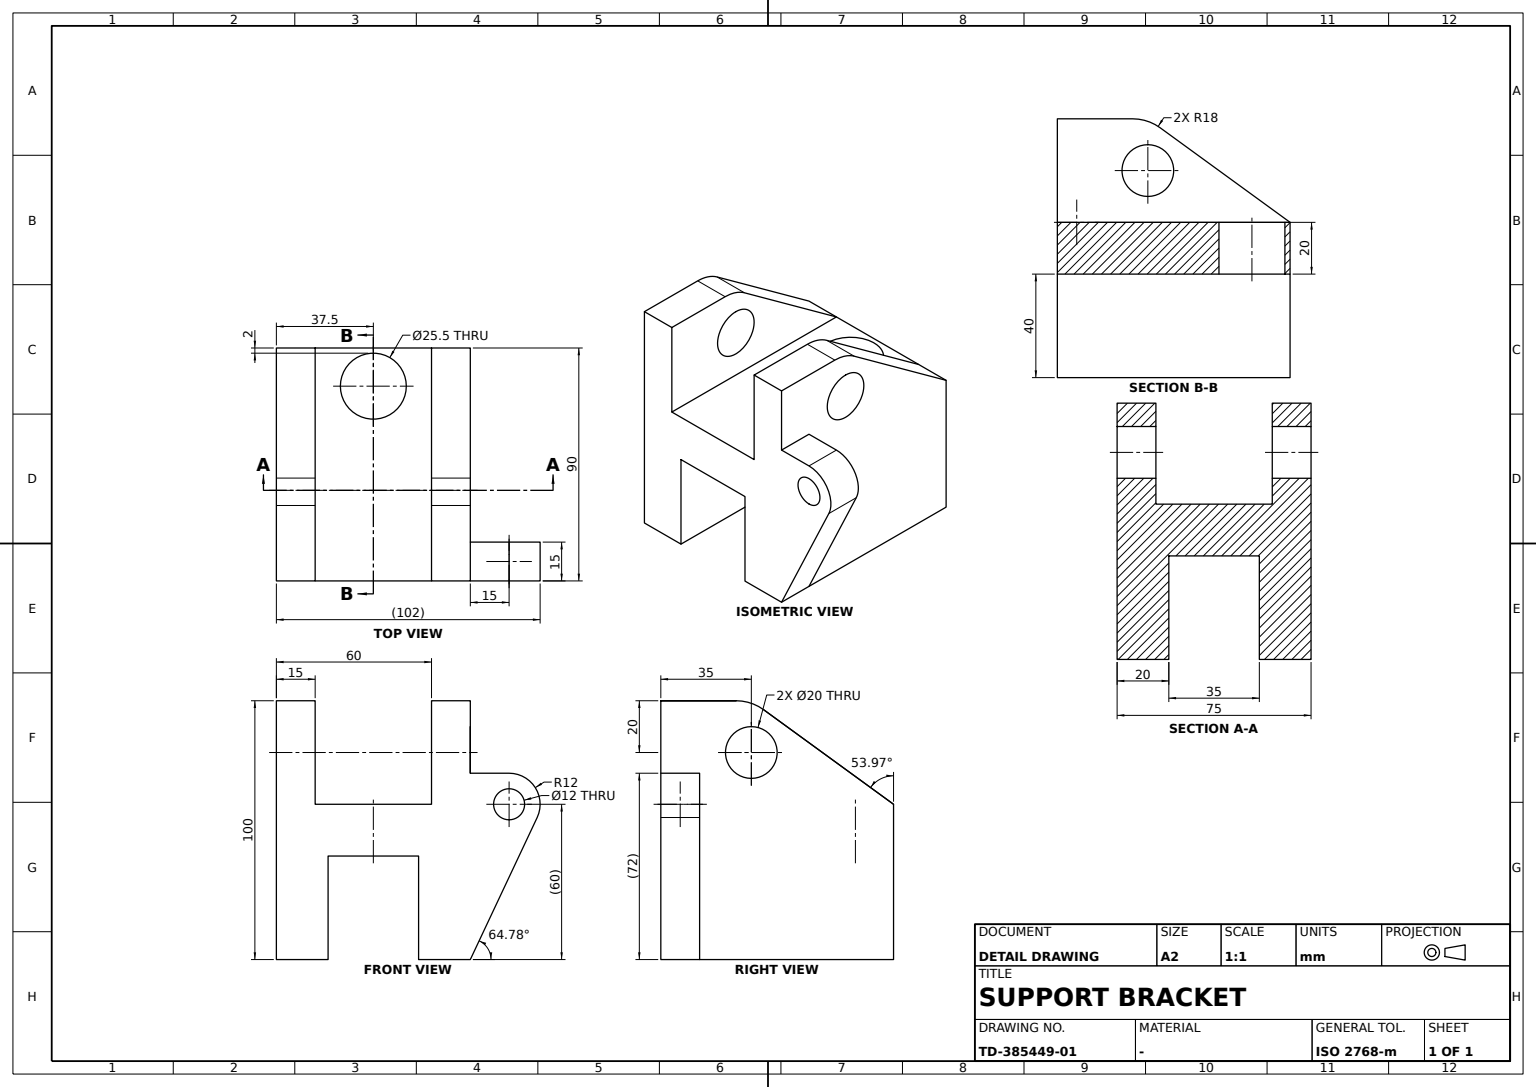
CATIA V5 part; units mm, degrees
sketch "Sketch1" plane through (0, 0, 0) normal (0, 1, 0) x (-1, 0, 0)
  line L0 (37.5, 30) -> (37.5, -30)
  line L1 (37.5, -30) -> (17.5, -30)
  line L2 (-37.5, -30) -> (-37.5, 30)
  line L3 (-37.5, 30) -> (37.5, 30)
  point P0 (37.5, -30)
  point P1 (-37.5, -30)
  point P2 (0, -30)
  line L4 (17.5, -30) -> (17.5, 10)
  line L5 (17.5, 10) -> (-17.5, 10)
  line L6 (-17.5, 10) -> (-17.5, -30)
  point P3 (-17.5, -30)
  line L7 (-17.5, -30) -> (-37.5, -30)
  dimension "distance L1 L3" = 60
  dimension "distance L0 L2" = 75
  dimension "length L4" = 40
  dimension "length L5" = 35
  constraint vertical L0 y-axis
  constraint vertical L2 y-axis
  constraint vertical L4 y-axis
  constraint vertical L6 y-axis
  constraint horizontal L1 x-axis
  constraint horizontal L3 x-axis
  constraint horizontal L5 x-axis
  constraint horizontal L7 x-axis
  constraint equidistance L0 L2 origin
  constraint equidistance L1 L3 origin
  constraint equidistance P0 P1 P2
  constraint coincidence P3 L1
  constraint coincidence L1 P2
  constraint coincidence L1 L7
extrude "Pad1" add sketch "Sketch1" along normal blind 90
sketch "Sketch2" plane through (37.5, 0, 0) normal (1, 0, 0) x (0, 1, 0)
  line L0 (0, 30) -> (90, 30)
  line L1 (0, 30) -> (0, 50)
  point P0 (0, 50)
  circle A0 centre (35, 50) radius 10
  point P1 (0, 50)
  line L2 (0, 70) -> (0, 50)
  line L3 (0, 70) -> (35, 70)
  line L4 (35, 70) -> (90, 30)
  dimension "length L1" = 20
  dimension "radius A0" = 10
  constraint vertical L1 y-axis
  constraint horizontal L3 x-axis
  constraint coincidence P0 P1
extrude "Pad2" add sketch "Sketch2" against normal blind 15
fillet "Fillet1" radius 18 1 edges at (30, 35, 70)
sketch "Sketch3" plane through (-37.5, 0, 0) normal (-1, 0, 0) x (0, -1, 0)
  line L0 (0, 30) -> (0, 70)
  line L1 (0, 70) -> (-35, 70)
  line L2 (-35, 70) -> (-90, 30)
  line L3 (-90, 30) -> (0, 30)
  circle A0 centre (-35, 50) radius 10
  dimension "length L0" = 40
  dimension "length L1" = 35
  dimension "radius A0" = 10
  dimension "distance A0 L1" = 10
  constraint vertical L0 y-axis
  constraint horizontal L1 x-axis
  constraint horizontal L3 x-axis
extrude "Pad3" add sketch "Sketch3" against normal blind 15
fillet "Fillet2" radius 18 1 edges at (-30, 35, 70)
sketch "Sketch4" plane through (0, 0, 0) normal (0, -1, 0) x (1, 0, 0)
  arc A0 (63.3558, 24.8861) -> (52.5, 42) centre (52.5, 30) ccw
  circle A1 centre (52.5, 30) radius 6
  line L0 (63.3558, 24.8861) -> (37.5, -30)
  line L1 (37.5, -30) -> (37.5, 42)
  line L2 (52.5, 42) -> (37.5, 42)
  dimension "radius A0" = 12
  dimension "radius A1" = 6
  constraint tangency L0 A0
  constraint tangency L2 A0
  constraint vertical L1 y-axis
extrude "Pad4" add sketch "Sketch4" against normal blind 15
sketch "Sketch5" plane through (0, 0, 30) normal (0, 0, 1) x (1, 0, 0)
  circle A0 centre (0, 75.25) radius 12.75
  point P0 (0, 75.25)
  line L0 (-37.5, 90) -> (37.5, 90) construction
  dimension "radius A0" = 12.75
  dimension "distance A0 L0" = 2
  constraint coincidence P0 y-axis
extrude "Pocket1" cut sketch "Sketch5" against normal through all
